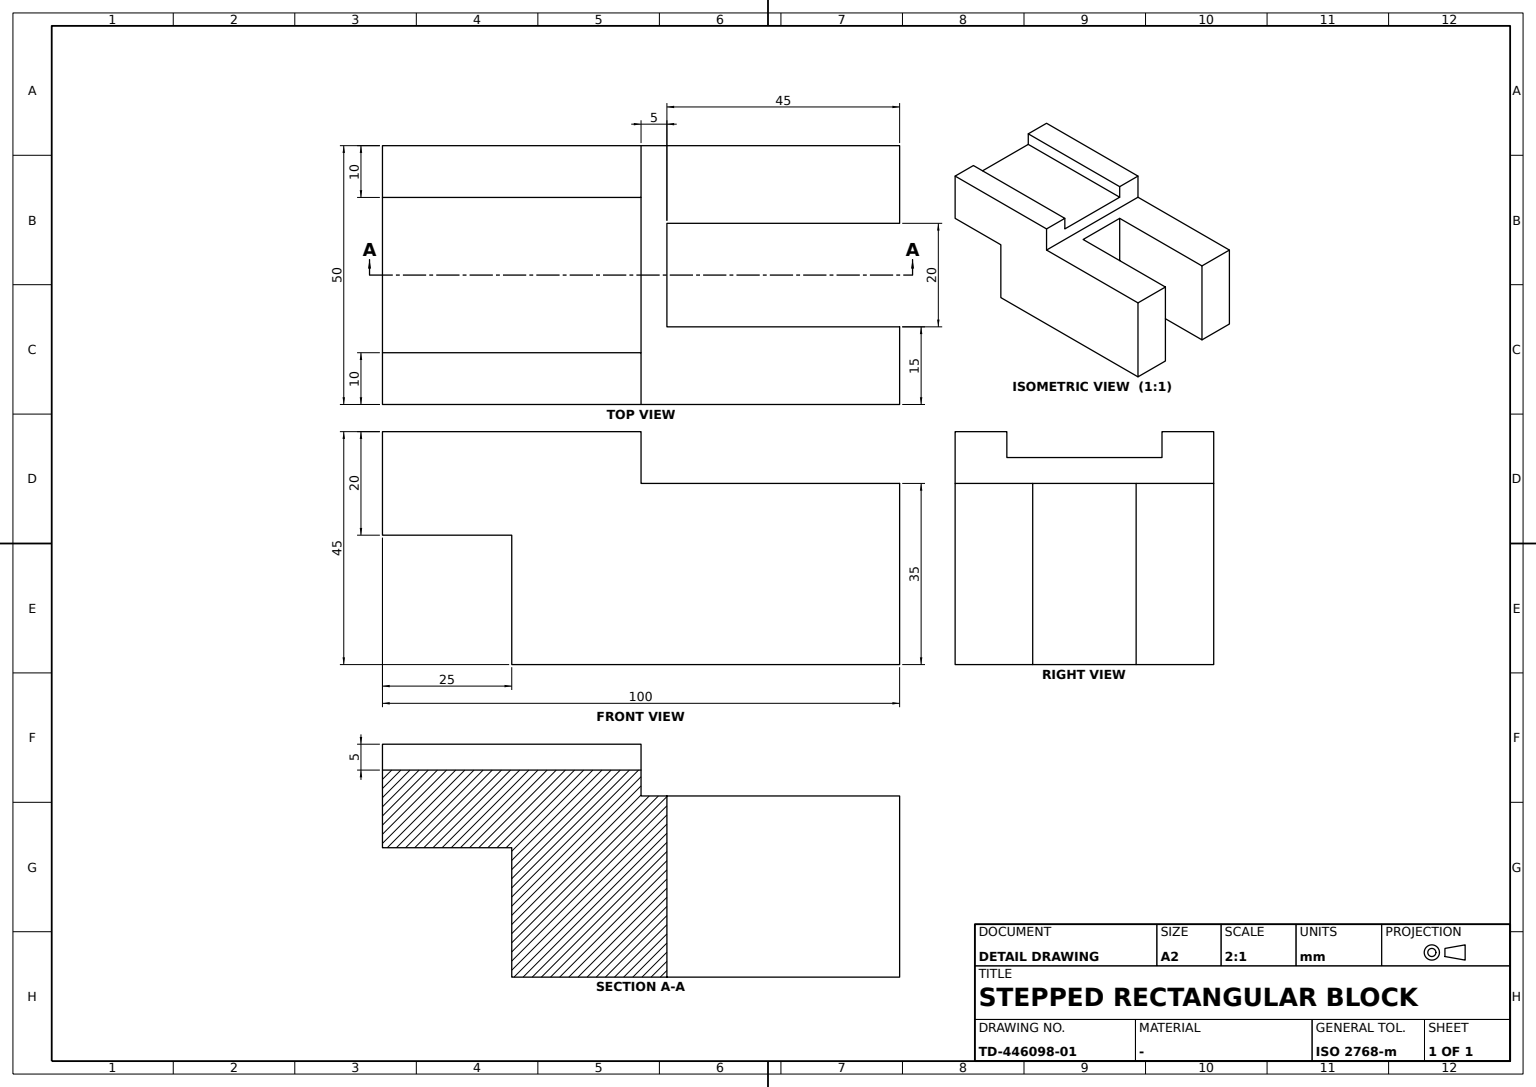
CATIA V5 part; units mm, degrees
sketch "Sketch1" plane through (0, 0, 0) normal (0, 1, 0) x (-1, 0, 0)
  line L0 (-50, 17.5) -> (-50, -17.5)
  line L1 (-50, -17.5) -> (50, -17.5)
  line L2 (50, -17.5) -> (50, 17.5)
  line L3 (50, 17.5) -> (-50, 17.5)
  dimension "length L0" = 35
  dimension "length L1" = 100
  constraint vertical L0 y-axis
  constraint vertical L2 y-axis
  constraint horizontal L1 x-axis
  constraint horizontal L3 x-axis
  constraint symmetry L0 L2 y-axis
  constraint symmetry L3 L1 x-axis
extrude "Pad1" add sketch "Sketch1" against normal blind 50
sketch "Sketch2" plane through (0, 0, 0) normal (1, 0, 0) x (0, 1, 0)
  point P0 (-50, 17.5)
  line L0 (-50, 17.5) -> (0, 17.5)
  point P1 (0, 17.5)
  line L1 (0, 17.5) -> (0, 27.5)
  line L2 (0, 27.5) -> (-10, 27.5)
  line L3 (-10, 27.5) -> (-10, 22.5)
  line L4 (-10, 22.5) -> (-40, 22.5)
  line L5 (-40, 22.5) -> (-40, 27.5)
  point P2 (-40, 27.5)
  line L6 (-40, 27.5) -> (-50, 27.5)
  line L7 (-50, 27.5) -> (-50, 17.5)
  point P3 (-50, 17.5)
  line L8 (0, 17.5) -> (-50, 17.5) construction
  point P4 (-50, 17.5)
  dimension "length L1" = 10
  dimension "length L2" = 10
  dimension "length L6" = 10
  dimension "length L5" = 5
  constraint coincidence P1 y-axis
  constraint coincidence P2 L2
  constraint coincidence P3 P0
  constraint coincidence L0 L8
  constraint coincidence P0 P4
  constraint horizontal L0 x-axis
  constraint horizontal L2 x-axis
  constraint horizontal L4 x-axis
  constraint horizontal L6 x-axis
  constraint vertical L1 y-axis
  constraint vertical L3 y-axis
  constraint vertical L5 y-axis
  constraint vertical L7 y-axis
extrude "Pad2" add sketch "Sketch2" against normal blind 50
sketch "Sketch3" plane through (0, 0, 0) normal (0, 1, 0) x (-1, 0, 0)
  line L0 (25, 7.5) -> (50, 7.5)
  line L1 (50, 7.5) -> (50, -17.5)
  line L2 (50, -17.5) -> (25, -17.5)
  line L3 (25, -17.5) -> (25, 7.5)
  line L4 (50, -17.5) -> (50, 17.5) construction
  line L5 (-50, -17.5) -> (50, -17.5) construction
  line L6 (0, 27.5) -> (50, 27.5) construction
  dimension "distance L6 L0" = 20
  constraint horizontal L0 x-axis
  constraint horizontal L2 x-axis
  constraint vertical L1 y-axis
  constraint vertical L3 y-axis
  constraint coincidence L1 L4
  constraint coincidence L5 L2
extrude "Pocket1" cut sketch "Sketch3" against normal blind 50
sketch "Sketch4" plane through (50, 0, 0) normal (1, 0, 0) x (0, 1, 0)
  line L0 (0, -17.5) -> (-50, -17.5) construction
  line L1 (-15, -17.5) -> (-35, -17.5)
  point P0 (-35, -17.5)
  line L2 (-35, -17.5) -> (-35, 17.5)
  line L3 (-35, 17.5) -> (-15, 17.5)
  line L4 (-15, 17.5) -> (-15, -17.5)
  point P1 (-15, -17.5)
  line L5 (0, 17.5) -> (0, -17.5) construction
  dimension "length L2" = 35
  dimension "length L3" = 20
  dimension "distance L4 L5" = 15
  constraint coincidence P0 L0
  constraint coincidence P1 L0
  constraint vertical L2 y-axis
  constraint vertical L4 y-axis
  constraint horizontal L3 x-axis
extrude "Pocket2" cut sketch "Sketch4" against normal blind 45
